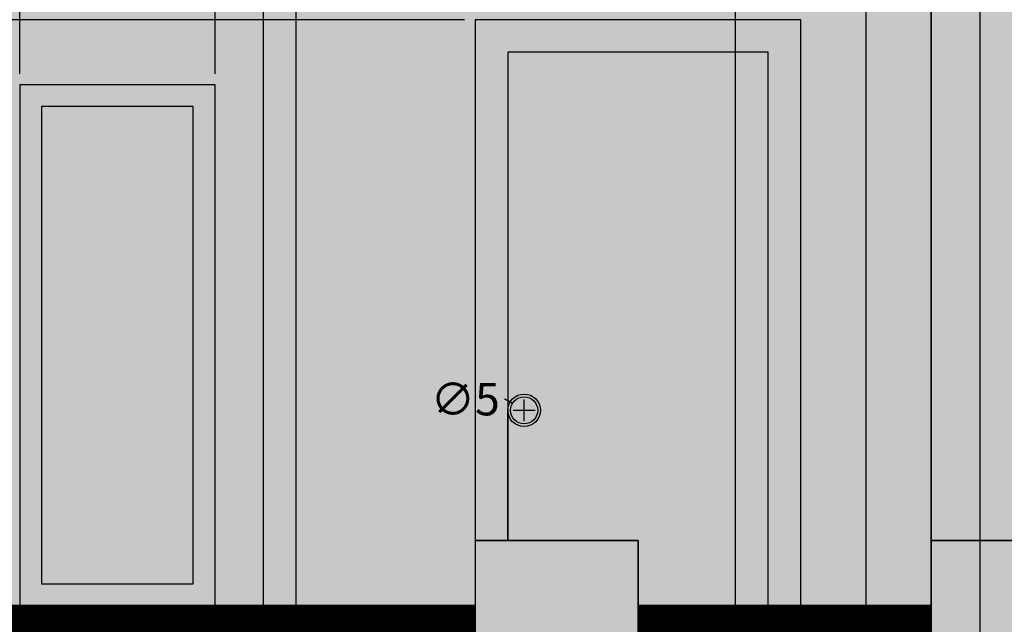
# Model space of a CAD drawing. Units: inches. Extents: x 860 to 1491, y 583 to 1370.
# Tile 3 of 8: x 1034 to 1216, y 727 to 839. Entities that reach past the tile are written whole.
import ezdxf

# ---------------------------------------------------------------- set-up
doc = ezdxf.new("R2010")
doc.units = ezdxf.units.IN
doc.header["$MEASUREMENT"] = 0
doc.layers.get('0').update_dxf_attribs({"color": 250})
for name, color, linetype, lineweight in [('A-ANNO-DIMS', 2, 'Continuous', 18), ('A-DOOR', 4, 'Continuous', 25), ('A-ELEV', 7, 'Continuous', 35), ('A-ELEV-PATT', 9, 'Continuous', 13), ('A-GLAZ', 4, 'Continuous', 25), ('A-GLAZ-PATT', 150, 'Continuous', 13), ('A-SITE-PATT', 8, 'Continuous', 13), ('A-SITE-WALL', 7, 'Continuous', 35)]:
    doc.layers.add(name, color=color, linetype=linetype, lineweight=lineweight)
doc.styles.get("Standard").update_dxf_attribs({"font": 'arial.ttf'})
doc.dimstyles.get("Standard").update_dxf_attribs({"dimtxt": 6, "dimasz": 0.18, "dimexe": 3, "dimexo": 2, "dimgap": 2, "dimtad": 0, "dimtih": 1, "dimtoh": 1, "dimdec": 0, "dimzin": 0, "dimdsep": 46, "dimlunit": 3, "dimtxsty": 'Standard', "dimblk2": 'CLOSEDBLANK', "dimsah": 1, "dimcen": 2, "dimadec": 0, "dimazin": 0, "dimtfac": 1, "dimtdec": 0, "dimtofl": 0, "dimtmove": 0, "dimatfit": 3, "dimfxl": 1, "dimtolj": 1, "dimtzin": 0, "dimarcsym": 0})

# ---------------------------------------------------------------- blocks, each defined once
blk = doc.blocks.new('_ClosedBlank')
at = {"color": 0, "linetype": 'ByBlock', "lineweight": -2}
for p, q in [((-1, 0.167), (0, 0)), ((-1, 0.167), (-1, -0.167)), ((0, 0), (-1, -0.167))]:
    blk.add_line(p, q, dxfattribs=at)
blk = doc.blocks.new('*D2')
at = {"layer": 'A-ANNO-DIMS', "color": 0, "lineweight": -2, "transparency": 16777216}
for p, q in [((1442.44, 1328.76), (1442.44, 584.11)), ((908.34, 740.76), (908.34, 584.11)), ((908.52, 587.11), (1163.85, 587.11)), ((1442.26, 587.11), (1186.93, 587.11))]:
    blk.add_line(p, q, dxfattribs=at)
at = {"layer": 'A-ANNO-DIMS', "color": 0, "transparency": 16777216}
blk.add_solid([(908.52, 587.14), (908.52, 587.08), (908.34, 587.11)], dxfattribs=at)
at = {"layer": 'Defpoints', "color": 0, "transparency": 16777216}
for p in [(1442.44, 1330.76), (908.34, 742.76), (1442.44, 587.11)]:
    blk.add_point(p, dxfattribs=at)
at = {"layer": 'A-ANNO-DIMS', "color": 0, "lineweight": -2, "transparency": 16777216, "xscale": 0.18, "yscale": 0.18, "zscale": 0.18}
blk.add_blockref('_ClosedBlank', (1442.44, 587.11), dxfattribs=at)
at = {"layer": 'A-ANNO-DIMS', "color": 0, "transparency": 16777216, "insert": (1175.39, 587.11), "char_height": 6, "attachment_point": 5}
blk.add_mtext('\\A1;534.1', dxfattribs=at)
blk = doc.blocks.new('*D12')
at = {"layer": 'A-ANNO-DIMS', "color": 0, "lineweight": -2, "transparency": 16777216}
for p, q in [((1118.44, 740.76), (1118.44, 584.11)), ((1112.44, 722.76), (1112.44, 584.11)), ((1112.62, 587.11), (1118.26, 587.11)), ((1118.44, 587.11), (1118.62, 587.11))]:
    blk.add_line(p, q, dxfattribs=at)
at = {"layer": 'A-ANNO-DIMS', "color": 0, "transparency": 16777216}
blk.add_solid([(1112.62, 587.14), (1112.62, 587.08), (1112.44, 587.11)], dxfattribs=at)
at = {"layer": 'Defpoints', "color": 0, "transparency": 16777216}
for p in [(1118.44, 742.76), (1112.44, 724.76), (1118.44, 587.11)]:
    blk.add_point(p, dxfattribs=at)
at = {"layer": 'A-ANNO-DIMS', "color": 0, "lineweight": -2, "transparency": 16777216, "xscale": 0.18, "yscale": 0.18, "zscale": 0.18}
blk.add_blockref('_ClosedBlank', (1118.44, 587.11), dxfattribs=at)
at = {"layer": 'A-ANNO-DIMS', "color": 0, "transparency": 16777216, "insert": (1122.6, 587.11), "char_height": 6, "attachment_point": 5}
blk.add_mtext('\\A1;6', dxfattribs=at)
blk = doc.blocks.new('*D13')
at = {"layer": 'A-ANNO-DIMS', "color": 0, "lineweight": -2, "transparency": 16777216}
for p, q in [((1118.44, 740.76), (1118.44, 584.11)), ((1148.44, 740.76), (1148.44, 584.11)), ((1118.62, 587.11), (1127.16, 587.11)), ((1148.26, 587.11), (1139.73, 587.11))]:
    blk.add_line(p, q, dxfattribs=at)
at = {"layer": 'A-ANNO-DIMS', "color": 0, "transparency": 16777216}
blk.add_solid([(1118.62, 587.14), (1118.62, 587.08), (1118.44, 587.11)], dxfattribs=at)
at = {"layer": 'Defpoints', "color": 0, "transparency": 16777216}
for p in [(1118.44, 742.76), (1148.44, 742.76), (1148.44, 587.11)]:
    blk.add_point(p, dxfattribs=at)
at = {"layer": 'A-ANNO-DIMS', "color": 0, "lineweight": -2, "transparency": 16777216, "xscale": 0.18, "yscale": 0.18, "zscale": 0.18}
blk.add_blockref('_ClosedBlank', (1148.44, 587.11), dxfattribs=at)
at = {"layer": 'A-ANNO-DIMS', "color": 0, "transparency": 16777216, "insert": (1133.44, 587.11), "char_height": 6, "attachment_point": 5}
blk.add_mtext('\\A1;30', dxfattribs=at)
blk = doc.blocks.new('*D14')
at = {"layer": 'A-ANNO-DIMS', "color": 0, "lineweight": -2, "transparency": 16777216}
for p, q in [((1148.44, 740.76), (1148.44, 584.11)), ((1154.44, 722.76), (1154.44, 584.11)), ((1148.62, 587.11), (1154.26, 587.11)), ((1154.44, 587.11), (1154.62, 587.11))]:
    blk.add_line(p, q, dxfattribs=at)
at = {"layer": 'A-ANNO-DIMS', "color": 0, "transparency": 16777216}
blk.add_solid([(1148.62, 587.14), (1148.62, 587.08), (1148.44, 587.11)], dxfattribs=at)
at = {"layer": 'Defpoints', "color": 0, "transparency": 16777216}
for p in [(1148.44, 742.76), (1154.44, 724.76), (1154.44, 587.11)]:
    blk.add_point(p, dxfattribs=at)
at = {"layer": 'A-ANNO-DIMS', "color": 0, "lineweight": -2, "transparency": 16777216, "xscale": 0.18, "yscale": 0.18, "zscale": 0.18}
blk.add_blockref('_ClosedBlank', (1154.44, 587.11), dxfattribs=at)
at = {"layer": 'A-ANNO-DIMS', "color": 0, "transparency": 16777216, "insert": (1158.6, 587.11), "char_height": 6, "attachment_point": 5}
blk.add_mtext('\\A1;6', dxfattribs=at)
blk = doc.blocks.new('*D16')
at = {"layer": 'A-ANNO-DIMS', "color": 0, "lineweight": -2, "transparency": 16777216}
for p, q in [((1202.44, 740.76), (1202.44, 584.11)), ((1196.44, 722.76), (1196.44, 584.11)), ((1196.62, 587.11), (1202.26, 587.11)), ((1202.44, 587.11), (1202.62, 587.11))]:
    blk.add_line(p, q, dxfattribs=at)
at = {"layer": 'A-ANNO-DIMS', "color": 0, "transparency": 16777216}
blk.add_solid([(1196.62, 587.14), (1196.62, 587.08), (1196.44, 587.11)], dxfattribs=at)
at = {"layer": 'Defpoints', "color": 0, "transparency": 16777216}
for p in [(1202.44, 742.76), (1196.44, 724.76), (1202.44, 587.11)]:
    blk.add_point(p, dxfattribs=at)
at = {"layer": 'A-ANNO-DIMS', "color": 0, "lineweight": -2, "transparency": 16777216, "xscale": 0.18, "yscale": 0.18, "zscale": 0.18}
blk.add_blockref('_ClosedBlank', (1202.44, 587.11), dxfattribs=at)
at = {"layer": 'A-ANNO-DIMS', "color": 0, "transparency": 16777216, "insert": (1206.6, 587.11), "char_height": 6, "attachment_point": 5}
blk.add_mtext('\\A1;6', dxfattribs=at)
blk = doc.blocks.new('*D17')
at = {"layer": 'A-ANNO-DIMS', "color": 0, "lineweight": -2, "transparency": 16777216}
for p, q in [((1202.44, 740.76), (1202.44, 584.11)), ((1232.44, 740.76), (1232.44, 584.11)), ((1202.62, 587.11), (1211.16, 587.11)), ((1232.26, 587.11), (1223.73, 587.11))]:
    blk.add_line(p, q, dxfattribs=at)
at = {"layer": 'A-ANNO-DIMS', "color": 0, "transparency": 16777216}
blk.add_solid([(1202.62, 587.14), (1202.62, 587.08), (1202.44, 587.11)], dxfattribs=at)
at = {"layer": 'Defpoints', "color": 0, "transparency": 16777216}
for p in [(1202.44, 742.76), (1232.44, 742.76), (1232.44, 587.11)]:
    blk.add_point(p, dxfattribs=at)
at = {"layer": 'A-ANNO-DIMS', "color": 0, "lineweight": -2, "transparency": 16777216, "xscale": 0.18, "yscale": 0.18, "zscale": 0.18}
blk.add_blockref('_ClosedBlank', (1232.44, 587.11), dxfattribs=at)
at = {"layer": 'A-ANNO-DIMS', "color": 0, "transparency": 16777216, "insert": (1217.44, 587.11), "char_height": 6, "attachment_point": 5}
blk.add_mtext('\\A1;30', dxfattribs=at)
blk = doc.blocks.new('*D22')
at = {"layer": 'A-ANNO-DIMS', "color": 0, "lineweight": -2, "transparency": 16777216}
for p, q in [((1034.46, 828.76), (1034.46, 1369.41)), ((1070.46, 828.76), (1070.46, 1369.41)), ((1034.64, 1366.41), (1046.17, 1366.41)), ((1070.28, 1366.41), (1058.75, 1366.41))]:
    blk.add_line(p, q, dxfattribs=at)
at = {"layer": 'A-ANNO-DIMS', "color": 0, "transparency": 16777216}
blk.add_solid([(1034.64, 1366.44), (1034.64, 1366.38), (1034.46, 1366.41)], dxfattribs=at)
at = {"layer": 'Defpoints', "color": 0, "transparency": 16777216}
for p in [(1070.46, 1366.41), (1034.46, 826.76), (1070.46, 826.76)]:
    blk.add_point(p, dxfattribs=at)
at = {"layer": 'A-ANNO-DIMS', "color": 0, "lineweight": -2, "transparency": 16777216, "xscale": 0.18, "yscale": 0.18, "zscale": 0.18}
blk.add_blockref('_ClosedBlank', (1070.46, 1366.41), dxfattribs=at)
at = {"layer": 'A-ANNO-DIMS', "color": 0, "transparency": 16777216, "insert": (1052.46, 1366.41), "char_height": 6, "attachment_point": 5}
blk.add_mtext('\\A1;36', dxfattribs=at)
blk = doc.blocks.new('*D23')
at = {"layer": 'A-ANNO-DIMS', "color": 0, "lineweight": -2, "transparency": 16777216}
for p, q in [((1070.46, 828.76), (1070.46, 1369.41)), ((1118.44, 840.76), (1118.44, 1369.41)), ((1070.64, 1366.41), (1082.2, 1366.41)), ((1118.26, 1366.41), (1106.7, 1366.41))]:
    blk.add_line(p, q, dxfattribs=at)
at = {"layer": 'A-ANNO-DIMS', "color": 0, "transparency": 16777216}
blk.add_solid([(1070.64, 1366.44), (1070.64, 1366.38), (1070.46, 1366.41)], dxfattribs=at)
at = {"layer": 'Defpoints', "color": 0, "transparency": 16777216}
for p in [(1118.44, 1366.41), (1118.44, 838.76), (1070.46, 826.76)]:
    blk.add_point(p, dxfattribs=at)
at = {"layer": 'A-ANNO-DIMS', "color": 0, "lineweight": -2, "transparency": 16777216, "xscale": 0.18, "yscale": 0.18, "zscale": 0.18}
blk.add_blockref('_ClosedBlank', (1118.44, 1366.41), dxfattribs=at)
at = {"layer": 'A-ANNO-DIMS', "color": 0, "transparency": 16777216, "insert": (1094.45, 1366.41), "char_height": 6, "attachment_point": 5}
blk.add_mtext('\\A1;47.98', dxfattribs=at)
blk = doc.blocks.new('*D25')
at = {"layer": 'A-ANNO-DIMS', "color": 0, "lineweight": -2, "transparency": 16777216}
for p, q in [((1178.44, 840.76), (1178.44, 1369.41)), ((1202.44, 744.76), (1202.44, 1369.41)), ((1178.62, 1366.41), (1184.1, 1366.41)), ((1202.26, 1366.41), (1196.78, 1366.41))]:
    blk.add_line(p, q, dxfattribs=at)
at = {"layer": 'A-ANNO-DIMS', "color": 0, "transparency": 16777216}
blk.add_solid([(1178.62, 1366.44), (1178.62, 1366.38), (1178.44, 1366.41)], dxfattribs=at)
at = {"layer": 'Defpoints', "color": 0, "transparency": 16777216}
for p in [(1202.44, 1366.41), (1178.44, 838.76), (1202.44, 742.76)]:
    blk.add_point(p, dxfattribs=at)
at = {"layer": 'A-ANNO-DIMS', "color": 0, "lineweight": -2, "transparency": 16777216, "xscale": 0.18, "yscale": 0.18, "zscale": 0.18}
blk.add_blockref('_ClosedBlank', (1202.44, 1366.41), dxfattribs=at)
at = {"layer": 'A-ANNO-DIMS', "color": 0, "transparency": 16777216, "insert": (1190.44, 1366.41), "char_height": 6, "attachment_point": 5}
blk.add_mtext('\\A1;24', dxfattribs=at)
blk = doc.blocks.new('*D26')
at = {"layer": 'A-ANNO-DIMS', "color": 0, "lineweight": -2, "transparency": 16777216}
for p, q in [((1202.44, 744.76), (1202.44, 1369.41)), ((1268.44, 864.76), (1268.44, 1369.41)), ((1202.62, 1366.41), (1229.13, 1366.41)), ((1268.26, 1366.41), (1241.75, 1366.41))]:
    blk.add_line(p, q, dxfattribs=at)
at = {"layer": 'A-ANNO-DIMS', "color": 0, "transparency": 16777216}
blk.add_solid([(1202.62, 1366.44), (1202.62, 1366.38), (1202.44, 1366.41)], dxfattribs=at)
at = {"layer": 'Defpoints', "color": 0, "transparency": 16777216}
for p in [(1268.44, 1366.41), (1268.44, 862.76), (1202.44, 742.76)]:
    blk.add_point(p, dxfattribs=at)
at = {"layer": 'A-ANNO-DIMS', "color": 0, "lineweight": -2, "transparency": 16777216, "xscale": 0.18, "yscale": 0.18, "zscale": 0.18}
blk.add_blockref('_ClosedBlank', (1268.44, 1366.41), dxfattribs=at)
at = {"layer": 'A-ANNO-DIMS', "color": 0, "transparency": 16777216, "insert": (1235.44, 1366.41), "char_height": 6, "attachment_point": 5}
blk.add_mtext('\\A1;66', dxfattribs=at)
blk = doc.blocks.new('*D35')
at = {"layer": 'A-ANNO-DIMS', "color": 0, "lineweight": -2, "transparency": 16777216}
for p, q in [((1116.440309, 838.755507), (869.690309, 838.755507)), ((872.690309, 838.935507), (872.690309, 839.115507)), ((1032.458453, 826.755507), (869.690309, 826.755507)), ((872.690309, 826.575507), (872.690309, 826.395507))]:
    blk.add_line(p, q, dxfattribs=at)
at = {"layer": 'A-ANNO-DIMS', "color": 0, "transparency": 16777216}
blk.add_solid([(872.660309, 826.575507), (872.720309, 826.575507), (872.690309, 826.755507)], dxfattribs=at)
at = {"layer": 'Defpoints', "color": 0, "transparency": 16777216}
for p in [(872.690309, 838.755507), (1118.440309, 838.755507), (1034.458453, 826.755507)]:
    blk.add_point(p, dxfattribs=at)
at = {"layer": 'A-ANNO-DIMS', "color": 0, "lineweight": -2, "transparency": 16777216, "xscale": 0.18, "yscale": 0.18, "zscale": 0.18, "rotation": 270}
blk.add_blockref('_ClosedBlank', (872.690309, 838.755507), dxfattribs=at)
at = {"layer": 'A-ANNO-DIMS', "color": 0, "transparency": 16777216, "insert": (872.690309, 832.755507), "char_height": 6, "attachment_point": 5}
blk.add_mtext('\\A1;12', dxfattribs=at)
blk = doc.blocks.new('*D65')
at = {"layer": 'A-ANNO-DIMS', "color": 0, "lineweight": -2, "transparency": 16777216}
for p, q in [((998.34, 956.76), (998.34, 584.11)), ((1079.34, 956.76), (1079.34, 584.11)), ((998.52, 587.11), (1033.12, 587.11)), ((1079.16, 587.11), (1044.56, 587.11))]:
    blk.add_line(p, q, dxfattribs=at)
at = {"layer": 'A-ANNO-DIMS', "color": 0, "transparency": 16777216}
blk.add_solid([(998.52, 587.14), (998.52, 587.08), (998.34, 587.11)], dxfattribs=at)
at = {"layer": 'Defpoints', "color": 0, "transparency": 16777216}
for p in [(998.34, 958.76), (1079.34, 958.76), (1079.34, 587.11)]:
    blk.add_point(p, dxfattribs=at)
at = {"layer": 'A-ANNO-DIMS', "color": 0, "lineweight": -2, "transparency": 16777216, "xscale": 0.18, "yscale": 0.18, "zscale": 0.18}
blk.add_blockref('_ClosedBlank', (1079.34, 587.11), dxfattribs=at)
at = {"layer": 'A-ANNO-DIMS', "color": 0, "transparency": 16777216, "insert": (1038.84, 587.11), "char_height": 6, "attachment_point": 5}
blk.add_mtext('\\A1;81', dxfattribs=at)
blk = doc.blocks.new('*D66')
at = {"layer": 'A-ANNO-DIMS', "color": 0, "lineweight": -2, "transparency": 16777216}
for p, q in [((1079.34, 956.76), (1079.34, 584.11)), ((1085.34, 956.76), (1085.34, 584.11)), ((1079.52, 587.11), (1085.16, 587.11)), ((1085.34, 587.11), (1085.52, 587.11))]:
    blk.add_line(p, q, dxfattribs=at)
at = {"layer": 'A-ANNO-DIMS', "color": 0, "transparency": 16777216}
blk.add_solid([(1079.52, 587.14), (1079.52, 587.08), (1079.34, 587.11)], dxfattribs=at)
at = {"layer": 'Defpoints', "color": 0, "transparency": 16777216}
for p in [(1079.34, 958.76), (1085.34, 958.76), (1085.34, 587.11)]:
    blk.add_point(p, dxfattribs=at)
at = {"layer": 'A-ANNO-DIMS', "color": 0, "lineweight": -2, "transparency": 16777216, "xscale": 0.18, "yscale": 0.18, "zscale": 0.18}
blk.add_blockref('_ClosedBlank', (1085.34, 587.11), dxfattribs=at)
at = {"layer": 'A-ANNO-DIMS', "color": 0, "transparency": 16777216, "insert": (1089.5, 587.11), "char_height": 6, "attachment_point": 5}
blk.add_mtext('\\A1;6', dxfattribs=at)
blk = doc.blocks.new('*D67')
at = {"layer": 'A-ANNO-DIMS', "color": 0, "lineweight": -2, "transparency": 16777216}
for p, q in [((1085.34, 956.76), (1085.34, 584.11)), ((1166.34, 956.76), (1166.34, 584.11)), ((1085.52, 587.11), (1120.12, 587.11)), ((1166.16, 587.11), (1131.56, 587.11))]:
    blk.add_line(p, q, dxfattribs=at)
at = {"layer": 'A-ANNO-DIMS', "color": 0, "transparency": 16777216}
blk.add_solid([(1085.52, 587.14), (1085.52, 587.08), (1085.34, 587.11)], dxfattribs=at)
at = {"layer": 'Defpoints', "color": 0, "transparency": 16777216}
for p in [(1085.34, 958.76), (1166.34, 958.76), (1166.34, 587.11)]:
    blk.add_point(p, dxfattribs=at)
at = {"layer": 'A-ANNO-DIMS', "color": 0, "lineweight": -2, "transparency": 16777216, "xscale": 0.18, "yscale": 0.18, "zscale": 0.18}
blk.add_blockref('_ClosedBlank', (1166.34, 587.11), dxfattribs=at)
at = {"layer": 'A-ANNO-DIMS', "color": 0, "transparency": 16777216, "insert": (1125.84, 587.11), "char_height": 6, "attachment_point": 5}
blk.add_mtext('\\A1;81', dxfattribs=at)
blk = doc.blocks.new('*D68')
at = {"layer": 'A-ANNO-DIMS', "color": 0, "lineweight": -2, "transparency": 16777216}
for p, q in [((1211.44, 980.76), (1211.44, 584.11)), ((1166.34, 956.76), (1166.34, 584.11)), ((1166.52, 587.11), (1179.56, 587.11)), ((1211.26, 587.11), (1198.22, 587.11))]:
    blk.add_line(p, q, dxfattribs=at)
at = {"layer": 'A-ANNO-DIMS', "color": 0, "transparency": 16777216}
blk.add_solid([(1166.52, 587.14), (1166.52, 587.08), (1166.34, 587.11)], dxfattribs=at)
at = {"layer": 'Defpoints', "color": 0, "transparency": 16777216}
for p in [(1211.44, 982.76), (1166.34, 958.76), (1211.44, 587.11)]:
    blk.add_point(p, dxfattribs=at)
at = {"layer": 'A-ANNO-DIMS', "color": 0, "lineweight": -2, "transparency": 16777216, "xscale": 0.18, "yscale": 0.18, "zscale": 0.18}
blk.add_blockref('_ClosedBlank', (1211.44, 587.11), dxfattribs=at)
at = {"layer": 'A-ANNO-DIMS', "color": 0, "transparency": 16777216, "insert": (1188.89, 587.11), "char_height": 6, "attachment_point": 5}
blk.add_mtext('\\A1;45.1', dxfattribs=at)
blk = doc.blocks.new('*D69')
at = {"layer": 'A-ANNO-DIMS', "color": 0, "lineweight": -2, "transparency": 16777216}
for p, q in [((1211.440309, 980.755507), (1211.440309, 584.105507)), ((1220.440309, 896.755507), (1220.440309, 584.105507)), ((1211.260309, 587.105507), (1211.080309, 587.105507)), ((1220.620309, 587.105507), (1220.800309, 587.105507))]:
    blk.add_line(p, q, dxfattribs=at)
at = {"layer": 'A-ANNO-DIMS', "color": 0, "transparency": 16777216}
blk.add_solid([(1211.260309, 587.135507), (1211.260309, 587.075507), (1211.440309, 587.105507)], dxfattribs=at)
at = {"layer": 'Defpoints', "color": 0, "transparency": 16777216}
for p in [(1211.440309, 982.755507), (1220.440309, 898.755507), (1220.440309, 587.105507)]:
    blk.add_point(p, dxfattribs=at)
at = {"layer": 'A-ANNO-DIMS', "color": 0, "lineweight": -2, "transparency": 16777216, "xscale": 0.18, "yscale": 0.18, "zscale": 0.18, "rotation": 180}
blk.add_blockref('_ClosedBlank', (1220.440309, 587.105507), dxfattribs=at)
at = {"layer": 'A-ANNO-DIMS', "color": 0, "transparency": 16777216, "insert": (1215.940309, 587.105507), "char_height": 6, "attachment_point": 5}
blk.add_mtext('\\A1;9', dxfattribs=at)
blk = doc.blocks.new('*D76')
at = {"layer": 'A-ANNO-DIMS', "color": 0, "lineweight": -2, "transparency": 16777216}
for p, q in [((1202.440309, 1277.755507), (1202.440309, 584.105507)), ((1190.440309, 1214.755507), (1190.440309, 584.105507)), ((1190.260309, 587.105507), (1190.080309, 587.105507)), ((1202.620309, 587.105507), (1202.800309, 587.105507))]:
    blk.add_line(p, q, dxfattribs=at)
at = {"layer": 'A-ANNO-DIMS', "color": 0, "transparency": 16777216}
blk.add_solid([(1190.260309, 587.135507), (1190.260309, 587.075507), (1190.440309, 587.105507)], dxfattribs=at)
at = {"layer": 'Defpoints', "color": 0, "transparency": 16777216}
for p in [(1202.440309, 1279.755507), (1190.440309, 1216.755507), (1202.440309, 587.105507)]:
    blk.add_point(p, dxfattribs=at)
at = {"layer": 'A-ANNO-DIMS', "color": 0, "lineweight": -2, "transparency": 16777216, "xscale": 0.18, "yscale": 0.18, "zscale": 0.18, "rotation": 180}
blk.add_blockref('_ClosedBlank', (1202.440309, 587.105507), dxfattribs=at)
at = {"layer": 'A-ANNO-DIMS', "color": 0, "transparency": 16777216, "insert": (1196.440309, 587.105507), "char_height": 6, "attachment_point": 5}
blk.add_mtext('\\A1;12', dxfattribs=at)
blk = doc.blocks.new('*D77')
at = {"layer": 'A-ANNO-DIMS', "color": 0, "lineweight": -2, "transparency": 16777216}
for p, q in [((1202.44, 1277.76), (1202.44, 584.11)), ((1352.44, 1277.76), (1352.44, 584.11)), ((1202.62, 587.11), (1269.1, 587.11)), ((1352.26, 587.11), (1285.78, 587.11))]:
    blk.add_line(p, q, dxfattribs=at)
at = {"layer": 'A-ANNO-DIMS', "color": 0, "transparency": 16777216}
blk.add_solid([(1202.62, 587.14), (1202.62, 587.08), (1202.44, 587.11)], dxfattribs=at)
at = {"layer": 'Defpoints', "color": 0, "transparency": 16777216}
for p in [(1202.44, 1279.76), (1352.44, 1279.76), (1352.44, 587.11)]:
    blk.add_point(p, dxfattribs=at)
at = {"layer": 'A-ANNO-DIMS', "color": 0, "lineweight": -2, "transparency": 16777216, "xscale": 0.18, "yscale": 0.18, "zscale": 0.18}
blk.add_blockref('_ClosedBlank', (1352.44, 587.11), dxfattribs=at)
at = {"layer": 'A-ANNO-DIMS', "color": 0, "transparency": 16777216, "insert": (1277.44, 587.11), "char_height": 6, "attachment_point": 5}
blk.add_mtext('\\A1;150', dxfattribs=at)
blk = doc.blocks.new('*D87')
at = {"layer": 'A-ANNO-DIMS', "color": 0, "lineweight": -2, "transparency": 16777216}
for p, q in [((1123.83, 768.82), (1124.01, 768.82)), ((1124.01, 768.82), (1125.14, 768.14)), ((1127.44, 764.76), (1127.44, 768.76)), ((1125.44, 766.76), (1129.44, 766.76))]:
    blk.add_line(p, q, dxfattribs=at)
at = {"layer": 'Defpoints', "color": 0, "transparency": 16777216}
for p in [(1125.3, 768.04), (1129.58, 765.47)]:
    blk.add_point(p, dxfattribs=at)
at = {"layer": 'A-ANNO-DIMS', "color": 0, "lineweight": -2, "transparency": 16777216, "xscale": 0.18, "yscale": 0.18, "zscale": 0.18, "rotation": 328.9823293658701}
blk.add_blockref('_ClosedBlank', (1125.3, 768.04), dxfattribs=at)
at = {"layer": 'A-ANNO-DIMS', "color": 0, "transparency": 16777216, "insert": (1116.58, 768.82), "char_height": 6, "attachment_point": 5}
blk.add_mtext('\\A1;∅5', dxfattribs=at)

msp = doc.modelspace()

# ---------------------------------------------------------------- hatches: boundary and pattern name
at = {"layer": 'A-ELEV-PATT'}
h = msp.add_hatch(color=256, dxfattribs=at)
h.dxf.hatch_style = 1
h.paths.add_polyline_path([(1442.4403, 1330.7555), (1370.4403, 1330.7555), (1370.4403, 622.7555), (1442.4403, 622.7555)])
h.paths.add_polyline_path([(1358.4403, 1306.7555), (1190.4403, 1306.7555), (1190.4403, 1288.7555), (1358.4403, 1288.7555)])
h.paths.add_polyline_path([(1190.4403, 1234.7555), (962.3403, 1234.7555), (962.3403, 1198.7555), (1202.4403, 1198.7555), (1202.4403, 1216.7555), (1190.4403, 1216.7555)])
h.paths.add_polyline_path([(1202.4403, 1117.6207), (962.3403, 1117.6207), (962.3403, 982.7555), (986.3403, 982.7555), (986.3403, 1090.7555), (1178.3403, 1090.7555), (1178.3403, 982.7555), (1202.4403, 982.7555)])
h.paths.add_polyline_path([(1319.4403, 1184.7555), (1202.4403, 1184.7555), (1202.4403, 982.7555), (1211.4403, 982.7555), (1211.4403, 946.7555), (1220.4403, 946.7555), (1220.4403, 934.7555), (1319.4403, 934.7555)])
h.paths.add_polyline_path([(1271.4403, 1160.7555), (1307.4403, 1160.7555), (1307.4403, 944.7555), (1271.4403, 944.7555)], flags=16)
h.paths.add_polyline_path([(1275.4403, 1156.7555), (1303.4403, 1156.7555), (1303.4403, 948.7555), (1275.4403, 948.7555)], flags=0)
h.paths.add_polyline_path([(1202.4403, 898.7555), (962.3403, 898.7555), (962.3403, 730.7555), (1034.4585, 730.7555), (1034.4585, 826.7555), (1070.4585, 826.7555), (1070.4585, 730.7555), (1118.4403, 730.7555), (1118.4403, 838.7555), (1178.4403, 838.7555), (1178.4403, 730.7555), (1202.4403, 730.7555)])
h.paths.add_polyline_path([(1220.4403, 946.7555), (1211.4403, 946.7555), (938.3403, 946.7555), (926.3403, 946.7555), (926.3403, 910.7555), (962.3403, 910.7555), (1220.4403, 910.7555)])
h.paths.add_polyline_path([(950.3403, 730.7555), (950.3403, 734.7555), (938.3403, 742.7555), (938.3403, 730.7555), (938.3403, 622.7555), (950.3403, 622.7555)])
h = msp.add_hatch(color=256, dxfattribs=at)
h.dxf.hatch_style = 1
h.paths.add_polyline_path([(1352.4403, 1279.7555), (1202.4403, 1279.7555), (1202.4403, 1198.7555), (1328.4403, 1198.7555), (1328.4403, 922.7555), (1220.4403, 922.7555), (1220.4403, 898.7555), (1202.4403, 898.7555), (1202.4403, 742.7555), (1232.4403, 742.7555), (1232.4403, 730.7555), (1352.4403, 730.7555)])
h.paths.add_polyline_path([(1268.4403, 862.7555), (1340.4403, 862.7555), (1340.4403, 790.7555), (1268.4403, 790.7555)], flags=16)
h.paths.add_polyline_path([(1272.4403, 858.7555), (1302.4403, 858.7555), (1302.4403, 794.7555), (1272.4403, 794.7555)], flags=0)
h.paths.add_polyline_path([(1306.4403, 858.7555), (1336.4403, 858.7555), (1336.4403, 794.7555), (1306.4403, 794.7555)], flags=0)
h = msp.add_hatch(color=256, dxfattribs=at)
h.paths.add_polyline_path([(1176.3403, 1088.7555), (988.3403, 1088.7555), (988.3403, 982.7555), (998.3403, 982.7555), (998.3403, 1078.7555), (1079.3403, 1078.7555), (1079.3403, 982.7555), (1085.3403, 982.7555), (1085.3403, 1078.7555), (1166.3403, 1078.7555), (1166.3403, 982.7555), (1176.3403, 982.7555)])
h.paths.add_polyline_path([(1176.3403, 982.7555), (1166.3403, 982.7555), (1166.3403, 958.7555), (1085.3403, 958.7555), (1085.3403, 982.7555), (1079.3403, 982.7555), (1079.3403, 958.7555), (998.3403, 958.7555), (998.3403, 982.7555), (988.3403, 982.7555), (988.3403, 948.7555), (1176.3403, 948.7555)])
h.paths.add_polyline_path([(1307.4403, 1160.7555), (1271.4403, 1160.7555), (1271.4403, 944.7555), (1307.4403, 944.7555)])
h.paths.add_polyline_path([(1275.4403, 1156.7555), (1303.4403, 1156.7555), (1303.4403, 948.7555), (1275.4403, 948.7555)], flags=16)
h.paths.add_polyline_path([(1340.4403, 862.7555), (1268.4403, 862.7555), (1268.4403, 790.7555), (1340.4403, 790.7555)])
h.paths.add_polyline_path([(1306.4403, 794.7555), (1306.4403, 858.7555), (1336.4403, 858.7555), (1336.4403, 794.7555)], flags=16)
h.paths.add_polyline_path([(1302.4403, 794.7555), (1272.4403, 794.7555), (1272.4403, 858.7555), (1302.4403, 858.7555)], flags=16)
h.paths.add_polyline_path([(1124.4403, 832.7555), (1172.4403, 832.7555), (1172.4403, 730.7555), (1178.4403, 730.7555), (1178.4403, 838.7555), (1118.4403, 838.7555), (1118.4403, 742.7555), (1124.4403, 742.7555), (1124.4403, 766.7555)])
h.paths.add_polyline_path([(1070.4585, 826.7555), (1034.4585, 826.7555), (1034.4585, 730.7555), (1070.4585, 730.7555)])
h.paths.add_polyline_path([(1066.4585, 822.7555), (1066.4585, 734.7555), (1038.4585, 734.7555), (1038.4585, 822.7555)], flags=16)
h.paths.add_polyline_path([(1129.9403, 766.7555, 1), (1124.9403, 766.7555, 1)], flags=17)
h = msp.add_hatch(color=256, dxfattribs=at)
h.dxf.hatch_style = 1
h.paths.add_polyline_path([(1370.4403, 730.7555), (1232.4403, 730.7555), (1232.4403, 622.7555), (1370.4403, 622.7555)])
h.paths.add_polyline_path([(1232.4403, 730.7555), (1232.4403, 742.7555), (1202.4403, 742.7555), (1202.4403, 622.7555), (1232.4403, 622.7555)])
h.paths.add_polyline_path([(1148.4403, 730.7555), (1148.4403, 742.7555), (1118.4403, 742.7555), (1118.4403, 718.7555), (1118.4403, 622.7555), (1148.4403, 622.7555)])
h.paths.add_polyline_path([(938.3403, 730.7555), (938.3403, 742.7555), (908.3403, 742.7555), (908.3403, 736.7555), (908.3403, 622.7555), (938.3403, 622.7555)])
at = {"layer": 'A-GLAZ-PATT'}
h = msp.add_hatch(color=256, dxfattribs=at)
h.paths.add_polyline_path([(1178.3403, 982.7555), (1176.3403, 982.7555), (1176.3403, 948.7555), (988.3403, 948.7555), (988.3403, 982.7555), (986.3403, 982.7555), (986.3403, 946.7555), (1178.3403, 946.7555)])
h.paths.add_polyline_path([(1178.3403, 1090.7555), (986.3403, 1090.7555), (986.3403, 982.7555), (988.3403, 982.7555), (988.3403, 1088.7555), (1176.3403, 1088.7555), (1176.3403, 982.7555), (1178.3403, 982.7555)])
h.paths.add_polyline_path([(1124.4403, 766.7555, 1), (1130.4403, 766.7555, 1)])
h.paths.add_polyline_path([(1129.9403, 766.7555, -1), (1124.9403, 766.7555, -1)], flags=16)
h = msp.add_hatch(color=256, dxfattribs=at)
h.set_gradient(color1=(153, 27, 30), color2=(153, 38, 0), name='INVCYLINDER')
h.paths.add_polyline_path([(1172.4403, 832.7555), (1124.4403, 832.7555), (1124.4403, 766.7555, -1), (1130.4403, 766.7555, -1), (1124.4403, 766.7555), (1124.4403, 742.7555), (1148.4403, 742.7555), (1148.4403, 730.7555), (1172.4403, 730.7555)])
h = msp.add_hatch(color=256, dxfattribs=at)
h.set_gradient(color1=(51, 167, 230), color2=(122, 175, 223), name='CYLINDER')
h.paths.add_polyline_path([(1066.4585, 822.7555), (1038.4585, 822.7555), (1038.4585, 734.7555), (1066.4585, 734.7555)])
at = {"layer": 'A-SITE-PATT'}
h = msp.add_hatch(dxfattribs=at)
h.set_pattern_fill('GRAVEL', color=256, scale=30, style=0)
h.set_pattern_definition([(228.01279, (21.6, 30), (-240, -270), [4.0361, -399.57264]), (184.96974, (18.9, 27), (360, 30), [6.92604, -685.67774]), (132.51045, (12, 26.4), (300, -330), [4.88364, -483.481]), (267.27369, (0.3, 18.9), (30, 600), [6.30714, -624.40674]), (292.83365, (0, 12.6), (-150, 360), [6.18465, -612.2812]), (357.27369, (2.4, 6.9), (-600, 30), [6.30714, -624.40674]), (37.69424, (8.7, 6.6), (-390, -300), [8.34087, -825.74546]), (72.25533, (15.3, 11.7), (210, 660), [7.87464, -779.58964]), (121.42957, (17.7, 19.2), (-240, 390), [6.3285, -626.5222]), (175.23636, (14.4, 24.6), (330, -30), [7.22496, -354.0229]), (222.39744, (7.2, 25.2), (-360, -330), [9.34344, -925.00125]), (138.81407, (30, 18.6), (-210, 180), [3.18903, -315.71534]), (171.46923, (27.6, 20.7), (390, -60), [6.0671, -600.64534]), (225, (21.6, 21.6), (-3e-15, -30), [4.24263, -38.1838]), (203.1986, (19.5, 25.2), (150, 60), [2.28474, -226.18845]), (291.8014, (17.4, 24.3), (-30, 90), [3.2311, -158.32385]), (30.96376, (18.6, 21.3), (90, 60), [5.24787, -169.6807]), (161.56505, (23.1, 24), (60, -30), [3.79473, -91.0736]), (16.38954, (0, 24.3), (300, 90), [5.316, -526.28535]), (70.34618, (5.1, 25.8), (-120, -330), [4.45983, -441.52223]), (293.1986, (23.1, 30), (-60, 150), [4.56945, -223.90374]), (343.61046, (24.9, 25.8), (-300, 90), [5.316, -526.28535]), (339.44395, (0, 5.7), (-150, 60), [5.1264, -251.1937]), (294.77514, (4.8, 3.9), (-150, 330), [4.29534, -425.2393]), (66.8014, (23.4, 0), (60, 150), [4.56945, -223.90374]), (17.35402, (25.2, 4.2), (-390, -120), [5.02893, -497.8627]), (69.44395, (8.7, 0), (-60, -150), [2.5632, -253.7569]), (101.30993, (21.6, 0), (-30, 120), [1.5297, -151.4409]), (165.96376, (21.3, 1.5), (90, -30), [6.18465, -117.5085]), (186.00901, (15.3, 3), (300, 30), [5.7315, -567.4177]), (303.69007, (18.6, 18.6), (-30, 60), [4.32666, -103.8399]), (353.15723, (21, 15), (510, -60), [7.55382, -747.82688]), (60.9454, (28.5, 14.1), (-120, -210), [3.0887, -305.7802]), (90, (30, 16.8), (-30, 30), [1.8, -28.2]), (120.25644, (14.7, 3.9), (120, -210), [4.1677, -412.6056]), (48.01279, (12.6, 7.5), (240, 270), [8.07216, -395.53656]), (0, (18, 13.5), (30, 30), [7.8, -22.2]), (325.30485, (25.8, 13.5), (300, -210), [4.7434, -469.59823]), (254.0546, (29.7, 10.8), (-30, -120), [4.36806, -214.03524]), (207.64598, (28.5, 6.6), (-570, -300), [7.11195, -704.08423]), (175.42608, (22.2, 3.3), (-390, 30), [7.52397, -744.8722])])
h.paths.add_polyline_path([(1370.4403, 730.7555), (1232.4403, 730.7555), (1232.4403, 622.7555), (1370.4403, 622.7555)])
h.paths.add_polyline_path([(1232.4403, 730.7555), (1232.4403, 742.7555), (1202.4403, 742.7555), (1202.4403, 622.7555), (1232.4403, 622.7555)])
h.paths.add_polyline_path([(1148.4403, 730.7555), (1148.4403, 742.7555), (1118.4403, 742.7555), (1118.4403, 718.7555), (1118.4403, 622.7555), (1148.4403, 622.7555)])
h.paths.add_polyline_path([(938.3403, 730.7555), (938.3403, 742.7555), (908.3403, 742.7555), (908.3403, 736.7555), (908.3403, 622.7555), (938.3403, 622.7555)])
h = msp.add_hatch(dxfattribs=at)
h.set_pattern_fill('ANSI31', color=256, style=0)
h.paths.add_polyline_path([(1118.4403, 730.7555), (962.3403, 730.7555), (950.3403, 730.7555), (950.3403, 622.7555), (1118.4403, 622.7555)])
h.paths.add_polyline_path([(1028.4544, 724.7555), (1028.3903, 628.7074), (956.3403, 628.7555), (956.3403, 724.7555)], flags=16)
h.paths.add_polyline_path([(1040.4544, 724.7555), (1112.4403, 724.7555), (1112.4403, 628.7555), (1040.3903, 628.7555)], flags=16)
h.paths.add_polyline_path([(1202.4403, 730.7555), (1148.4403, 730.7555), (1148.4403, 622.7555), (1202.4403, 622.7555)])
h.paths.add_polyline_path([(1154.4403, 724.7555), (1196.4403, 724.7555), (1196.4403, 628.7555), (1154.4403, 628.7555)], flags=16)

# ---------------------------------------------------------------- linework, layer by layer
at = {"layer": 'A-DOOR'}
for p, q in [((1178.4403, 838.7555), (1118.4403, 838.7555)), ((1118.4403, 838.7555), (1118.4403, 718.7555)), ((1178.4403, 730.7555), (1178.4403, 838.7555)), ((1172.4403, 832.7555), (1124.4403, 832.7555)), ((1124.4403, 832.7555), (1124.4403, 742.7555)), ((1172.4403, 730.7555), (1172.4403, 832.7555)), ((1124.4403, 742.7555), (1124.4403, 766.7555))]:
    msp.add_line(p, q, dxfattribs=at)
for radius in [3, 2.5]:
    msp.add_circle((1127.4403, 766.7555), radius, dxfattribs=at)
at = {"layer": 'A-ELEV'}
for p, q in [((1202.4403, 622.7555), (1202.4403, 898.7555)), ((1232.4403, 742.7555), (1202.4403, 742.7555))]:
    msp.add_line(p, q, dxfattribs=at)
at = {"layer": 'A-GLAZ'}
for points in [[(1070.4585, 826.7555), (1034.4585, 826.7555), (1034.4585, 730.7555), (1070.4585, 730.7555)], [(1066.4585, 822.7555), (1038.4585, 822.7555), (1038.4585, 734.7555), (1066.4585, 734.7555)]]:
    msp.add_lwpolyline(points, close=True, dxfattribs=at)
at = {"layer": 'A-SITE-WALL'}
for p, q in [((1148.4403, 742.7555), (1118.4403, 742.7555)), ((1148.4403, 730.7555), (1148.4403, 742.7555)), ((962.3403, 730.7555), (1118.4403, 730.7555)), ((1118.4403, 730.7555), (1118.4403, 622.7555)), ((1148.4403, 730.7555), (1148.4403, 622.7555)), ((1148.4403, 730.7555), (1202.4403, 730.7555))]:
    msp.add_line(p, q, dxfattribs=at)

# ---------------------------------------------------------------- dimensions: what is measured, and where the dimension line sits
at = {"layer": 'A-ANNO-DIMS'}
for base, p1, p2, override, picture, middle in [((1070.4585, 1366.4055), (1034.4585, 826.7555), (1070.4585, 826.7555), {"dimdec": 0, "dimlfac": 1, "dimrnd": 0, "dimzin": 0, "dimdsep": 46, "dimlunit": 2}, '*D22', (1052.4585, 1366.4055)), ((1118.4403, 1366.4055), (1070.4585, 826.7555), (1118.4403, 838.7555), {"dimdec": 2, "dimlfac": 1, "dimrnd": 0, "dimzin": 0, "dimdsep": 46, "dimlunit": 2}, '*D23', (1094.4494, 1366.4055)), ((1202.4403, 1366.4055), (1178.4403, 838.7555), (1202.4403, 742.7555), {"dimdec": 0, "dimlfac": 1, "dimrnd": 0, "dimzin": 0, "dimdsep": 46, "dimlunit": 2}, '*D25', (1190.4403, 1366.4055)), ((1268.4403, 1366.4055), (1202.4403, 742.7555), (1268.4403, 862.7555), {"dimdec": 0, "dimlfac": 1, "dimrnd": 0, "dimzin": 0, "dimdsep": 46, "dimlunit": 2}, '*D26', (1235.4403, 1366.4055)), ((1442.4403, 587.1055), (908.3403, 742.7555), (1442.4403, 1330.7555), {"dimdec": 1, "dimlfac": 1, "dimrnd": 0, "dimzin": 0, "dimdsep": 46, "dimlunit": 2}, '*D2', (1175.3903, 587.1055)), ((1202.4403, 587.1055), (1190.4403, 1216.7555), (1202.4403, 1279.7555), {"dimdec": 0, "dimlfac": 1, "dimrnd": 0, "dimzin": 0, "dimdsep": 46, "dimlunit": 2}, '*D76', (1196.4403, 587.1055)), ((1352.4403, 587.1055), (1202.4403, 1279.7555), (1352.4403, 1279.7555), {"dimdec": 0, "dimlfac": 1, "dimrnd": 0, "dimzin": 0, "dimdsep": 46, "dimlunit": 2}, '*D77', (1277.4403, 587.1055)), ((1211.4403, 587.1055), (1166.3403, 958.7555), (1211.4403, 982.7555), {"dimdec": 1, "dimlfac": 1, "dimrnd": 0, "dimzin": 0, "dimdsep": 46, "dimlunit": 2}, '*D68', (1188.8903, 587.1055)), ((1220.4403, 587.1055), (1211.4403, 982.7555), (1220.4403, 898.7555), {"dimdec": 0, "dimlfac": 1, "dimrnd": 0, "dimzin": 0, "dimdsep": 46, "dimlunit": 2}, '*D69', (1215.9403, 587.1055)), ((1079.3403, 587.1055), (998.3403, 958.7555), (1079.3403, 958.7555), {"dimdec": 0, "dimlfac": 1, "dimrnd": 0, "dimzin": 0, "dimdsep": 46, "dimlunit": 2}, '*D65', (1038.8403, 587.1055)), ((1085.3403, 587.1055), (1079.3403, 958.7555), (1085.3403, 958.7555), {"dimdec": 0, "dimlfac": 1, "dimrnd": 0, "dimzin": 0, "dimdsep": 46, "dimlunit": 2}, '*D66', (1089.5012, 587.1055)), ((1166.3403, 587.1055), (1085.3403, 958.7555), (1166.3403, 958.7555), {"dimdec": 0, "dimlfac": 1, "dimrnd": 0, "dimzin": 0, "dimdsep": 46, "dimlunit": 2}, '*D67', (1125.8403, 587.1055)), ((1118.4403, 587.1055), (1112.4403, 724.7555), (1118.4403, 742.7555), {"dimdec": 0, "dimlfac": 1, "dimrnd": 0, "dimzin": 0, "dimdsep": 46, "dimlunit": 2}, '*D12', (1122.6012, 587.1055)), ((1148.4403, 587.1055), (1118.4403, 742.7555), (1148.4403, 742.7555), {"dimdec": 0, "dimlfac": 1, "dimrnd": 0, "dimzin": 0, "dimdsep": 46, "dimlunit": 2}, '*D13', (1133.4403, 587.1055)), ((1154.4403, 587.1055), (1148.4403, 742.7555), (1154.4403, 724.7555), {"dimdec": 0, "dimlfac": 1, "dimrnd": 0, "dimzin": 0, "dimdsep": 46, "dimlunit": 2}, '*D14', (1158.6012, 587.1055)), ((1202.4403, 587.1055), (1196.4403, 724.7555), (1202.4403, 742.7555), {"dimdec": 0, "dimlfac": 1, "dimrnd": 0, "dimzin": 0, "dimdsep": 46, "dimlunit": 2}, '*D16', (1206.6012, 587.1055)), ((1232.4403, 587.1055), (1202.4403, 742.7555), (1232.4403, 742.7555), {"dimdec": 0, "dimlfac": 1, "dimrnd": 0, "dimzin": 0, "dimdsep": 46, "dimlunit": 2}, '*D17', (1217.4403, 587.1055))]:
    dim = msp.add_linear_dim(base=base, p1=p1, p2=p2, dimstyle='Standard', override=override, dxfattribs=at)
    dim.commit()
    dim.dimension.update_dxf_attribs({"geometry": picture, "text_midpoint": middle})
dim = msp.add_linear_dim(base=(872.6903, 838.7555), p1=(1034.4585, 826.7555), p2=(1118.4403, 838.7555), angle=90, dimstyle='Standard', override={"dimdec": 0, "dimlfac": 1, "dimrnd": 0, "dimzin": 0, "dimdsep": 46, "dimlunit": 2}, dxfattribs=at)
dim.commit()
dim.dimension.update_dxf_attribs({"geometry": '*D35', "text_midpoint": (872.6903, 832.7555)})
dim = msp.add_diameter_dim_2p(p1=(1129.5828, 765.4673), p2=(1125.2978, 768.0438), dimstyle='Standard', override={"dimdec": 0, "dimlfac": 1, "dimrnd": 0, "dimzin": 0, "dimdsep": 46, "dimlunit": 2}, dxfattribs=at)
dim.commit()
dim.dimension.update_dxf_attribs({"geometry": '*D87', "text_midpoint": (1116.5792, 768.8167), "dimtype": 163})

doc.saveas('drawing.dxf')
